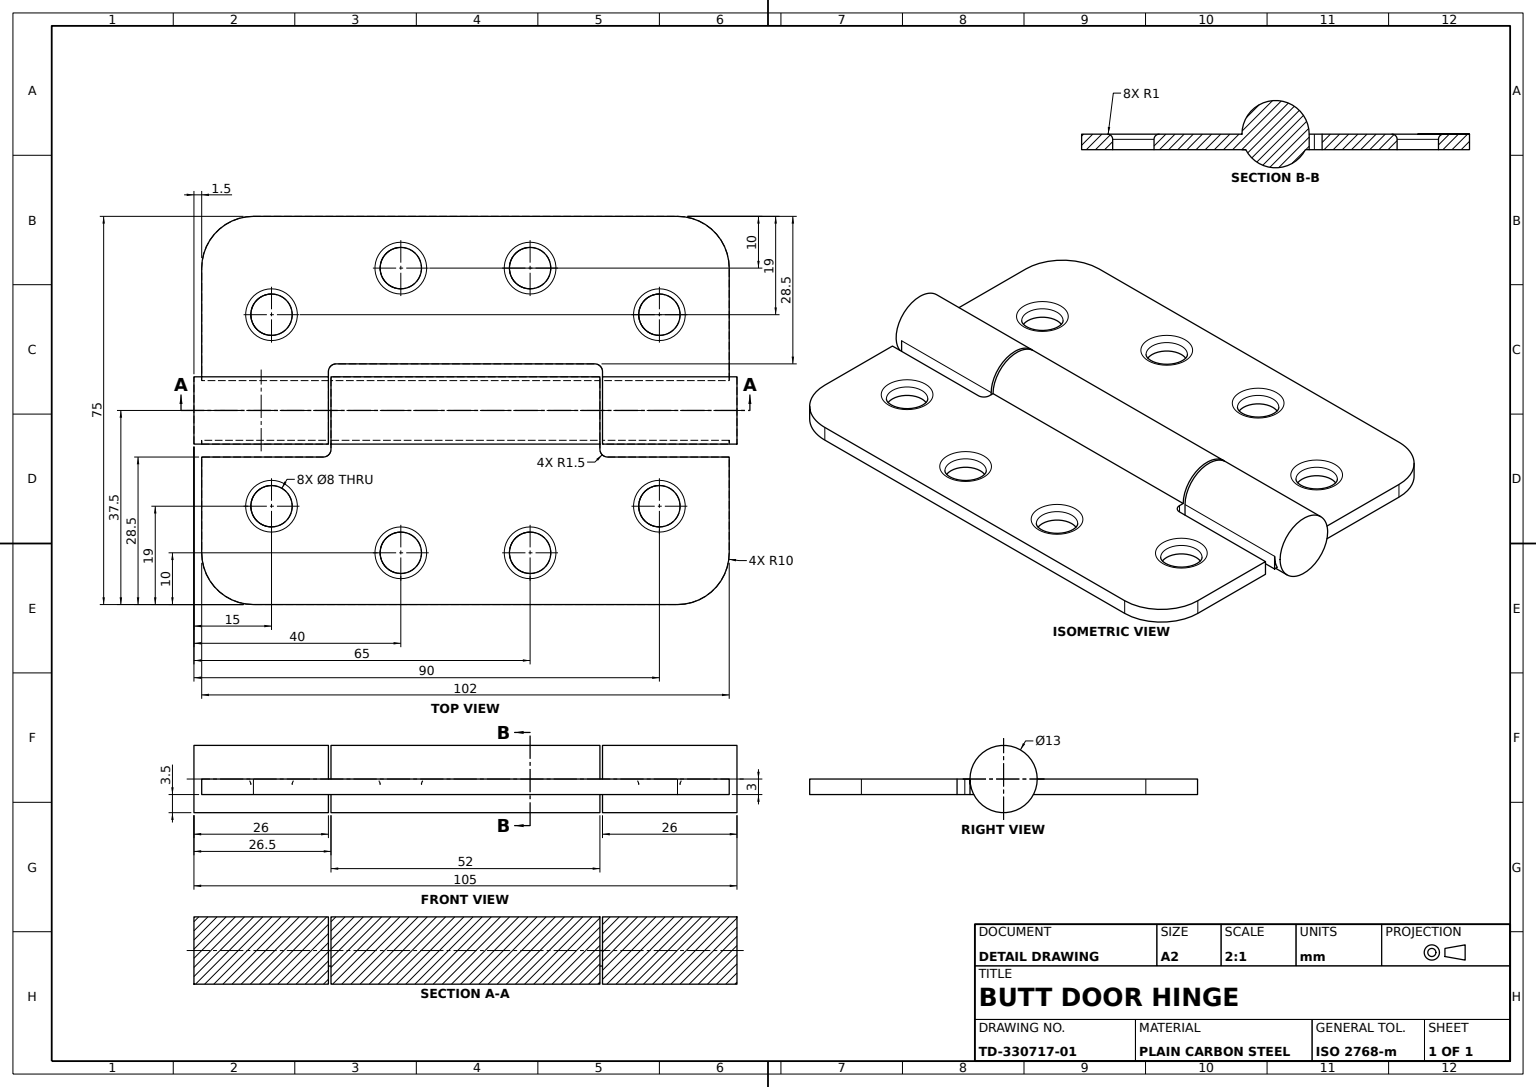
SolidWorks part; units mm, degrees
material "Plain Carbon Steel"
ref_plane "Front Plane" through (0, 0, 0) normal (0, 0, 1) x (1, 0, 0)
ref_plane "Top Plane" through (0, 0, 0) normal (0, 1, 0) x (1, 0, 0)
ref_plane "Right Plane" through (0, 0, 0) normal (1, 0, 0) x (0, 0, -1)
sketch "Hinge Leaves Profile" plane through (0, 0, 0) normal (0, 1, 0) x (1, 0, 0)
  line L0 (0, 0) -> (0, -6.5)
  line L1 (0, -6.5) -> (24.5, -6.5)
  line L2 (24.5, -6.5) -> (24.5, 7.5)
  line L3 (26, 9) -> (76, 9)
  line L4 (77.5, 7.5) -> (77.5, -6.5)
  line L5 (77.5, -6.5) -> (102, -6.5)
  line L6 (102, -6.5) -> (102, 27.5)
  line L7 (92, 37.5) -> (10, 37.5)
  line L8 (0, 27.5) -> (0, 0)
  line L9 (0, -9) -> (23.5, -9)
  line L10 (0, -9) -> (0, -27.5)
  line L11 (10, -37.5) -> (92, -37.5)
  line L12 (102, -27.5) -> (102, -9)
  line L13 (102, -9) -> (78.5, -9)
  line L14 (25, -7.5) -> (25, 6.5)
  line L15 (25, 6.5) -> (77, 6.5)
  line L16 (77, 6.5) -> (77, -7.5)
  arc A0 (102, 27.5) -> (92, 37.5) centre (92, 27.5) ccw
  arc A1 (10, 37.5) -> (0, 27.5) centre (10, 27.5) ccw
  arc A2 (77.5, 7.5) -> (76, 9) centre (76, 7.5) ccw
  arc A3 (26, 9) -> (24.5, 7.5) centre (26, 7.5) ccw
  arc A4 (78.5, -9) -> (77, -7.5) centre (78.5, -7.5) cw
  arc A5 (23.5, -9) -> (25, -7.5) centre (23.5, -7.5) ccw
  arc A6 (92, -37.5) -> (102, -27.5) centre (92, -27.5) ccw
  arc A7 (10, -37.5) -> (0, -27.5) centre (10, -27.5) cw
  point P16 (77.5, 9)
  point P19 (24.5, 9)
  point P30 (77, -9)
  point P33 (25, -9)
  point P36 (102, -37.5)
  point P39 (0, -37.5)
  dimension "D1" = 10
  dimension "D8" = 37.5
  dimension "D9" = 1.5
  dimension "D15" = 6.5
  dimension "D16" = 1.5
  dimension "D17" = 10
  dimension "D2" = 28.5
  dimension "D3" = 0
  dimension "D4" = 24.5
  dimension "D5" = 15.5
  dimension "D6" = 53
  dimension "D7" = 24.5
  dimension "D10" = 75
  dimension "D11" = 28.5
  dimension "D12" = 28.5
  dimension "D13" = 25
  dimension "D14" = 25
extrude "Hinge Leaves 3mm" add sketch "Hinge Leaves Profile" against normal blind 3
sketch "Screw Holes Profile" plane through (0, 0, 0) normal (0, 1, 0) x (1, 0, 0)
  line L0 (26, 9) -> (76, 9) construction
  line L1 (77, 6.5) -> (25, 6.5) construction
  circle A0 centre (13.5, 18.5) radius 4
  circle A1 centre (38.5, 27.5) radius 4
  circle A2 centre (63.5, 27.5) radius 4
  circle A3 centre (88.5, 18.5) radius 4
  circle A4 centre (13.5, -18.5) radius 4
  circle A5 centre (38.5, -27.5) radius 4
  circle A6 centre (63.5, -27.5) radius 4
  circle A7 centre (88.5, -18.5) radius 4
  point P19 (51, 9)
  point P22 (51, 6.5)
  dimension "D1" = 8
  dimension "D2" = 8
  dimension "D3" = 8
  dimension "D4" = 8
  dimension "D5" = 8
  dimension "D6" = 8
  dimension "D7" = 8
  dimension "D8" = 8
  dimension "D9" = 18.5
  dimension "D10" = 37
  dimension "D11" = 18.5
  dimension "D12" = 37
  dimension "D13" = 37.5
  dimension "D14" = 75
  dimension "D15" = 37.5
  dimension "D16" = 75
  dimension "D17" = 12.5
  dimension "D18" = 25
  dimension "D19" = 27.5
  dimension "D20" = 27.5
  dimension "D21" = 12.5
  dimension "D22" = 25
  dimension "D23" = 27.5
  dimension "D24" = 27.5
extrude "Screw Holes 8xØ8" cut sketch "Screw Holes Profile" against normal blind 3
fillet "Screw Hole Edge Fillet R1 A" radius 1 4 edges at (88.5, 0, -14.5) (63.5, 0, -23.5) (38.5, 0, -23.5) (13.5, 0, -14.5)
fillet "Screw Hole Edge Fillet R1 B" radius 1 4 edges at (88.5, 0, 22.5) (63.5, 0, 31.5) (38.5, 0, 31.5) (13.5, 0, 22.5)
ref_plane "Hinge Axis Plane" through (0, 0, 0) normal (0, 0, 1) x (1, 0, 0)
sketch "End Knuckle 1 Profile" plane through (0, 0, 0) normal (0, 0, 1) x (1, 0, 0)
  line L1 (24.5, 0) -> (-1.5, 0)
  line L2 (24.5, 0) -> (24.5, 6.5)
  line L3 (24.5, 6.5) -> (-1.5, 6.5)
  line L4 (-1.5, 0) -> (-1.5, 6.5)
  dimension "D1" = 26
  dimension "D2" = 6.5
revolve "End Knuckle 1 Ø13x26" add sketch "End Knuckle 1 Profile" angle 360 about L1
sketch "Centre Knuckle Profile" plane through (0, 0, 0) normal (0, 0, 1) x (1, 0, 0)
  line L1 (25, 0) -> (77, 0)
  line L2 (25, 0) -> (25, 6.5)
  line L3 (25, 6.5) -> (77, 6.5)
  line L4 (77, 0) -> (77, 6.5)
  dimension "D1" = 52
  dimension "D2" = 6.5
revolve "Centre Knuckle Ø13x52" add sketch "Centre Knuckle Profile" angle 360 about L1
sketch "End Knuckle 2 Profile" plane through (0, 0, 0) normal (0, 0, 1) x (1, 0, 0)
  line L1 (77.5, 0) -> (103.5, 0)
  line L2 (77.5, 0) -> (77.5, 6.5)
  line L3 (77.5, 6.5) -> (103.5, 6.5)
  line L4 (103.5, 0) -> (103.5, 6.5)
  dimension "D1" = 26
  dimension "D2" = 6.5
revolve "End Knuckle 2 Ø13x26" add sketch "End Knuckle 2 Profile" angle 360 about L1
